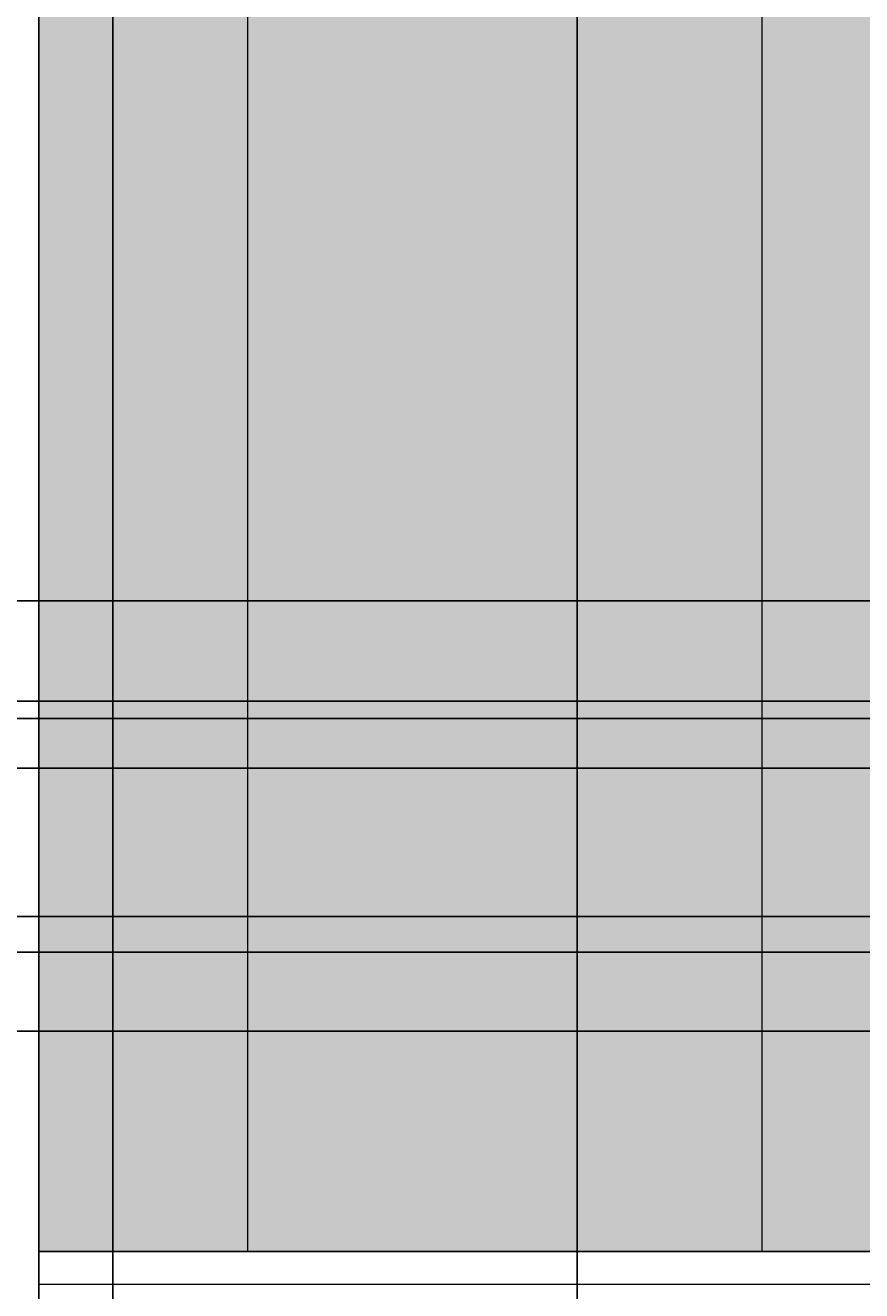
# Model space of a CAD drawing. Units: inches. Extents: x 36 to 594, y 79 to 831.
# Tile 17 of 30: x 93 to 189, y 446 to 590. Entities that reach past the tile are written whole.
import ezdxf

# ---------------------------------------------------------------- set-up
doc = ezdxf.new("R2010")
doc.units = ezdxf.units.IN
doc.header["$MEASUREMENT"] = 0
for name, color, linetype, lineweight in [('A-ANNO-DIMS', 2, 'Continuous', 18), ('A-ELEV', 7, 'Continuous', 25), ('A-ELEV-PATT', 8, 'Continuous', 13), ('A-GLAZ', 4, 'Continuous', 18)]:
    doc.layers.add(name, color=color, linetype=linetype, lineweight=lineweight)
doc.styles.get("Standard").update_dxf_attribs({"font": 'arial.ttf'})
doc.dimstyles.get("Standard").update_dxf_attribs({"dimtxt": 0.8125, "dimasz": 0.18, "dimexe": 0.18, "dimexo": 0.0625, "dimgap": 0.09, "dimtad": 0, "dimtih": 1, "dimtoh": 1, "dimdec": 4, "dimzin": 0, "dimdsep": 46, "dimlunit": 4, "dimtxsty": 'Standard', "dimcen": 0.09, "dimadec": 0, "dimazin": 0, "dimtfac": 1, "dimtdec": 4, "dimtofl": 0, "dimtmove": 0, "dimatfit": 3, "dimfxl": 1, "dimtolj": 1, "dimtzin": 0, "dimarcsym": 0})

# ---------------------------------------------------------------- blocks, each defined once
blk = doc.blocks.new('*D28')
at = {"layer": 'A-ANNO-DIMS', "color": 0, "lineweight": -2, "transparency": 16777216}
for p, q in [((269.3, 796.05), (37.49, 796.05)), ((37.67, 795.87), (37.67, 455.63)), ((37.67, 114.39), (37.67, 454.62)), ((94.8, 114.21), (37.49, 114.21))]:
    blk.add_line(p, q, dxfattribs=at)
at = {"layer": 'A-ANNO-DIMS', "color": 0, "transparency": 16777216}
for points in [[(37.64, 795.87), (37.7, 795.87), (37.67, 796.05)], [(37.64, 114.39), (37.7, 114.39), (37.67, 114.21)]]:
    blk.add_solid(points, dxfattribs=at)
at = {"layer": 'Defpoints', "color": 0, "transparency": 16777216}
for p in [(37.67, 796.05), (269.36, 796.05), (94.87, 114.21)]:
    blk.add_point(p, dxfattribs=at)
at = {"layer": 'A-ANNO-DIMS', "color": 0, "transparency": 16777216, "insert": (37.67, 455.13), "char_height": 0.812, "attachment_point": 5}
blk.add_mtext('\\A1;681.8', dxfattribs=at)
blk = doc.blocks.new('*D60')
at = {"layer": 'A-ANNO-DIMS', "color": 0, "lineweight": -2, "transparency": 16777216}
for p, q in [((103.34, 286.24), (103.34, 830.73)), ((103.52, 830.55), (128.41, 830.55)), ((156.23, 830.55), (131.33, 830.55)), ((156.41, 264.68), (156.41, 830.73))]:
    blk.add_line(p, q, dxfattribs=at)
at = {"layer": 'A-ANNO-DIMS', "color": 0, "transparency": 16777216}
for points in [[(103.52, 830.58), (103.52, 830.52), (103.34, 830.55)], [(156.23, 830.58), (156.23, 830.52), (156.41, 830.55)]]:
    blk.add_solid(points, dxfattribs=at)
at = {"layer": 'Defpoints', "color": 0, "transparency": 16777216}
for p in [(156.41, 830.55), (103.34, 286.18), (156.41, 264.62)]:
    blk.add_point(p, dxfattribs=at)
at = {"layer": 'A-ANNO-DIMS', "color": 0, "transparency": 16777216, "insert": (129.87, 830.55), "char_height": 0.812, "attachment_point": 5}
blk.add_mtext('\\A1;53.07', dxfattribs=at)
blk = doc.blocks.new('*D61')
at = {"layer": 'A-ANNO-DIMS', "color": 0, "lineweight": -2, "transparency": 16777216}
for p, q in [((156.41, 264.68), (156.41, 830.73)), ((156.59, 830.55), (185.26, 830.55)), ((216.85, 830.55), (188.18, 830.55)), ((217.03, 286.24), (217.03, 830.73))]:
    blk.add_line(p, q, dxfattribs=at)
at = {"layer": 'A-ANNO-DIMS', "color": 0, "transparency": 16777216}
for points in [[(156.59, 830.58), (156.59, 830.52), (156.41, 830.55)], [(216.85, 830.58), (216.85, 830.52), (217.03, 830.55)]]:
    blk.add_solid(points, dxfattribs=at)
at = {"layer": 'Defpoints', "color": 0, "transparency": 16777216}
for p in [(217.03, 830.55), (217.03, 286.18), (156.41, 264.62)]:
    blk.add_point(p, dxfattribs=at)
at = {"layer": 'A-ANNO-DIMS', "color": 0, "transparency": 16777216, "insert": (186.72, 830.55), "char_height": 0.812, "attachment_point": 5}
blk.add_mtext('\\A1;60.62', dxfattribs=at)
blk = doc.blocks.new('*D99')
at = {"layer": 'A-ANNO-DIMS', "color": 0, "lineweight": -2, "transparency": 16777216}
for p, q in [((236.23, 484.42), (37.49, 484.42)), ((37.67, 484.24), (37.67, 480.42)), ((37.67, 475.59), (37.67, 479.41)), ((232.76, 475.41), (37.49, 475.41))]:
    blk.add_line(p, q, dxfattribs=at)
at = {"layer": 'A-ANNO-DIMS', "color": 0, "transparency": 16777216}
for points in [[(37.64, 484.24), (37.7, 484.24), (37.67, 484.42)], [(37.64, 475.59), (37.7, 475.59), (37.67, 475.41)]]:
    blk.add_solid(points, dxfattribs=at)
at = {"layer": 'Defpoints', "color": 0, "transparency": 16777216}
for p in [(37.67, 484.42), (236.29, 484.42), (232.82, 475.41)]:
    blk.add_point(p, dxfattribs=at)
at = {"layer": 'A-ANNO-DIMS', "color": 0, "transparency": 16777216, "insert": (37.67, 479.92), "char_height": 0.812, "attachment_point": 5}
blk.add_mtext('\\A1;9.005', dxfattribs=at)
blk = doc.blocks.new('*D100')
at = {"layer": 'A-ANNO-DIMS', "color": 0, "lineweight": -2, "transparency": 16777216}
for p, q in [((236.23, 488.49), (37.49, 488.49)), ((37.67, 488.31), (37.67, 486.96)), ((37.67, 484.6), (37.67, 485.95)), ((236.23, 484.42), (37.49, 484.42))]:
    blk.add_line(p, q, dxfattribs=at)
at = {"layer": 'A-ANNO-DIMS', "color": 0, "transparency": 16777216}
for points in [[(37.64, 488.31), (37.7, 488.31), (37.67, 488.49)], [(37.64, 484.6), (37.7, 484.6), (37.67, 484.42)]]:
    blk.add_solid(points, dxfattribs=at)
at = {"layer": 'Defpoints', "color": 0, "transparency": 16777216}
for p in [(37.67, 488.49), (236.29, 488.49), (236.29, 484.42)]:
    blk.add_point(p, dxfattribs=at)
at = {"layer": 'A-ANNO-DIMS', "color": 0, "transparency": 16777216, "insert": (37.67, 486.46), "char_height": 0.812, "attachment_point": 5}
blk.add_mtext('\\A1;4.074', dxfattribs=at)
blk = doc.blocks.new('*D101')
at = {"layer": 'A-ANNO-DIMS', "color": 0, "lineweight": -2, "transparency": 16777216}
for p, q in [((236.23, 505.45), (37.49, 505.45)), ((37.67, 505.27), (37.67, 497.48)), ((37.67, 488.67), (37.67, 496.47)), ((236.23, 488.49), (37.49, 488.49))]:
    blk.add_line(p, q, dxfattribs=at)
at = {"layer": 'A-ANNO-DIMS', "color": 0, "transparency": 16777216}
for points in [[(37.64, 505.27), (37.7, 505.27), (37.67, 505.45)], [(37.64, 488.67), (37.7, 488.67), (37.67, 488.49)]]:
    blk.add_solid(points, dxfattribs=at)
at = {"layer": 'Defpoints', "color": 0, "transparency": 16777216}
for p in [(37.67, 505.45), (236.29, 505.45), (236.29, 488.49)]:
    blk.add_point(p, dxfattribs=at)
at = {"layer": 'A-ANNO-DIMS', "color": 0, "transparency": 16777216, "insert": (37.67, 496.97), "char_height": 0.812, "attachment_point": 5}
blk.add_mtext('\\A1;16.957', dxfattribs=at)
blk = doc.blocks.new('*D102')
at = {"layer": 'A-ANNO-DIMS', "color": 0, "lineweight": -2, "transparency": 16777216}
for p, q in [((232.76, 511.12), (37.49, 511.12)), ((37.67, 510.94), (37.67, 508.79)), ((37.67, 505.63), (37.67, 507.78)), ((236.23, 505.45), (37.49, 505.45))]:
    blk.add_line(p, q, dxfattribs=at)
at = {"layer": 'A-ANNO-DIMS', "color": 0, "transparency": 16777216}
for points in [[(37.64, 510.94), (37.7, 510.94), (37.67, 511.12)], [(37.64, 505.63), (37.7, 505.63), (37.67, 505.45)]]:
    blk.add_solid(points, dxfattribs=at)
at = {"layer": 'Defpoints', "color": 0, "transparency": 16777216}
for p in [(37.67, 511.12), (232.82, 511.12), (236.29, 505.45)]:
    blk.add_point(p, dxfattribs=at)
at = {"layer": 'A-ANNO-DIMS', "color": 0, "transparency": 16777216, "insert": (37.67, 508.29), "char_height": 0.812, "attachment_point": 5}
blk.add_mtext('\\A1;5.672', dxfattribs=at)
blk = doc.blocks.new('*D103')
at = {"layer": 'A-ANNO-DIMS', "color": 0, "lineweight": -2, "transparency": 16777216}
for p, q in [((232.76, 513.12), (37.49, 513.12)), ((37.67, 512.94), (37.67, 512.62)), ((232.76, 511.12), (37.49, 511.12)), ((37.67, 511.3), (37.67, 511.62))]:
    blk.add_line(p, q, dxfattribs=at)
at = {"layer": 'A-ANNO-DIMS', "color": 0, "transparency": 16777216}
for points in [[(37.64, 512.94), (37.7, 512.94), (37.67, 513.12)], [(37.64, 511.3), (37.7, 511.3), (37.67, 511.12)]]:
    blk.add_solid(points, dxfattribs=at)
at = {"layer": 'Defpoints', "color": 0, "transparency": 16777216}
for p in [(37.67, 513.12), (232.82, 513.12), (232.82, 511.12)]:
    blk.add_point(p, dxfattribs=at)
at = {"layer": 'A-ANNO-DIMS', "color": 0, "transparency": 16777216, "insert": (37.67, 512.12), "char_height": 0.812, "attachment_point": 5}
blk.add_mtext('\\A1;2', dxfattribs=at)
blk = doc.blocks.new('*D104')
at = {"layer": 'A-ANNO-DIMS', "color": 0, "lineweight": -2, "transparency": 16777216}
for p, q in [((232.76, 524.6), (37.49, 524.6)), ((37.67, 524.42), (37.67, 519.37)), ((37.67, 513.3), (37.67, 518.36)), ((232.76, 513.12), (37.49, 513.12))]:
    blk.add_line(p, q, dxfattribs=at)
at = {"layer": 'A-ANNO-DIMS', "color": 0, "transparency": 16777216}
for points in [[(37.64, 524.42), (37.7, 524.42), (37.67, 524.6)], [(37.64, 513.3), (37.7, 513.3), (37.67, 513.12)]]:
    blk.add_solid(points, dxfattribs=at)
at = {"layer": 'Defpoints', "color": 0, "transparency": 16777216}
for p in [(37.67, 524.6), (232.82, 524.6), (232.82, 513.12)]:
    blk.add_point(p, dxfattribs=at)
at = {"layer": 'A-ANNO-DIMS', "color": 0, "transparency": 16777216, "insert": (37.67, 518.86), "char_height": 0.812, "attachment_point": 5}
blk.add_mtext('\\A1;11.481', dxfattribs=at)

msp = doc.modelspace()

# ---------------------------------------------------------------- hatches: boundary and pattern name
at = {"layer": 'A-ELEV-PATT'}
h = msp.add_hatch(color=256, dxfattribs=at)
h.dxf.hatch_style = 1
h.paths.add_polyline_path([(398.0873, 796.0465), (269.3592, 796.0465), (269.3592, 770.1455), (397.8159, 770.1455)])
h.paths.add_polyline_path([(397.7518, 764.0341), (269.3592, 764.0341), (269.3592, 630.0394), (341.8367, 630.0394), (341.8367, 720.595), (335.0881, 728.3699), (329.982, 735.3373), (345.3661, 727.7743), (397.1052, 702.3389)])
h.paths.add_polyline_path([(341.8367, 594.2124), (201.4189, 594.2124), (201.4189, 475.4136), (232.8216, 475.4136), (232.8216, 524.6037), (341.8367, 524.6037)])
h.paths.add_polyline_path([(177.525, 594.2124), (118.7598, 594.2124), (118.7598, 450.2124), (177.525, 450.2124)])
h.paths.add_polyline_path([(424.4958, 594.2124), (365.7306, 594.2124), (365.7306, 450.2124), (424.4958, 450.2124)])
h.paths.add_polyline_path([(241.3553, 404.2737), (355.8569, 404.2737), (355.8569, 355.0836), (424.5492, 355.0836), (424.5492, 425.7333), (118.7598, 426.2844), (118.7598, 355.0836), (241.3553, 355.0836)])
h.paths.add_polyline_path([(448.3898, 306.2124), (217.0273, 306.2124), (217.0273, 142.2124), (254.0293, 142.2124), (254.0293, 150.9347), (254.0293, 286.1802), (401.5491, 286.1802), (401.5491, 150.9347), (401.5491, 142.2124), (448.3898, 142.2124)])
h.paths.add_polyline_path([(448.3898, 142.2124), (401.5491, 142.2124), (217.0273, 142.2124), (217.0273, 114.2124), (448.3898, 114.2124)])
h.paths.add_polyline_path([(217.0273, 306.2124), (174.7353, 306.2124), (94.8658, 306.2124), (94.8658, 162.2124), (103.3368, 162.2124), (103.3368, 264.6224), (103.3368, 286.1802), (217.0273, 286.1802)])
h = msp.add_hatch(color=256, dxfattribs=at)
h.dxf.hatch_style = 1
h.paths.add_polyline_path([(448.3898, 668.2124), (341.8367, 720.595), (341.8367, 594.2124), (341.8367, 450.2124), (365.7306, 450.2124), (365.7306, 594.2124), (424.4958, 594.2124), (424.4958, 450.2124), (448.3898, 450.2124), (448.3898, 594.2124)])
h.paths.add_polyline_path([(378.5958, 653.8563, -1), (413.2033, 653.8563, -1)], flags=16)
h.paths.add_polyline_path([(394.8995, 653.8563), (394.8995, 654.8563), (395.8995, 654.8563), (396.8995, 654.8563), (396.8995, 653.8563), (396.8995, 652.8563), (395.8995, 652.8563), (394.8995, 652.8563)], flags=0)
h.paths.add_polyline_path([(201.4189, 708.8485), (201.4189, 720.595), (94.8658, 668.2124), (94.8658, 644.2124), (94.8658, 596.2124), (94.8658, 594.2124), (94.8658, 450.2124), (118.7598, 450.2124), (118.7598, 594.2124), (177.525, 594.2124), (177.525, 450.2124), (201.4189, 450.2124), (201.4189, 594.2124)])
h.paths.add_polyline_path([(130.1589, 653.7648, -1), (164.7665, 653.7648, -1)], flags=16)
h.paths.add_polyline_path([(148.4627, 652.7648), (147.4627, 652.7648), (146.4627, 652.7648), (146.4627, 653.7648), (146.4627, 654.7648), (147.4627, 654.7648), (148.4627, 654.7648), (148.4627, 653.7648)], flags=0)
h = msp.add_hatch(dxfattribs=at)
h.set_pattern_fill('ANSI31', color=256, scale=38, angle=135)
h.paths.add_polyline_path([(448.3898, 450.2124), (94.8658, 450.2124), (94.8658, 306.2124), (174.7353, 306.2124), (448.3898, 306.2124), (448.3898, 367.5118)])
h.paths.add_polyline_path([(424.5492, 425.7333), (424.5492, 329.5325), (118.7598, 330.0836), (118.7598, 354.0836), (118.7598, 426.2844)], flags=16)
h.paths.add_polyline_path([(355.8569, 404.2737), (355.8569, 355.0836), (241.3553, 355.0836), (241.3553, 404.2737)], flags=0)
h.paths.add_polyline_path([(269.0393, 390.7924), (269.0393, 355.0836), (244.8248, 355.0836), (244.8248, 364.0887), (263.8892, 364.0887), (263.8892, 355.0836), (267.0393, 355.0836), (267.0393, 390.7924)], flags=0)
h.paths.add_polyline_path([(303.9765, 436.9126, -1), (313.1496, 436.9126, -1)], flags=16)
h.paths.add_polyline_path([(421.9473, 354.0836), (421.9376, 348.6883), (421.9376, 333.9204), (401.6342, 333.9204), (401.6705, 354.0836), (400.6705, 354.0836), (400.6608, 348.7267), (400.6608, 333.9587), (380.3574, 333.9587), (380.3937, 354.0836), (379.3937, 354.0836), (379.3841, 348.765), (379.3841, 333.997), (359.0807, 333.997), (359.1169, 354.0836), (358.1169, 354.0836), (358.1074, 348.8034), (358.1074, 334.0354), (337.804, 334.0354), (337.8401, 354.0836), (336.8401, 354.0836), (336.8306, 348.8417), (336.8306, 334.0737), (316.5272, 334.0737), (316.5633, 354.0836), (315.5633, 354.0836), (315.5539, 348.8801), (315.5539, 334.1121), (295.2505, 334.1121), (295.2865, 354.0836), (294.2865, 354.0836), (294.2772, 348.9184), (294.2772, 334.1504), (273.9738, 334.1504), (274.0097, 354.0836), (273.0097, 354.0836), (273.0005, 348.9568), (273.0005, 334.1888), (252.697, 334.1888), (252.7329, 354.0836), (251.7329, 354.0836), (251.7237, 348.9951), (251.7237, 334.2271), (231.4203, 334.2271), (231.4561, 354.0836), (230.4561, 354.0836), (230.447, 349.0335), (230.447, 334.2655), (210.1436, 334.2655), (210.1793, 354.0836), (209.1793, 354.0836), (209.1703, 349.0718), (209.1703, 334.3038), (188.8668, 334.3038), (188.9025, 354.0836), (187.9025, 354.0836), (187.8935, 349.1101), (187.8935, 334.3422), (167.5901, 334.3422), (167.6257, 354.0836), (166.6257, 354.0836), (166.6168, 349.1485), (166.6168, 334.3805), (146.3134, 334.3805), (146.3489, 354.0836), (145.3489, 354.0836), (145.3401, 349.1868), (145.3401, 334.4189), (125.0366, 334.4189), (125.0721, 354.0836)], flags=0)
h.paths.add_polyline_path([(266.285, 436.9126, -1), (275.458, 436.9126, -1)], flags=16)
h.paths.add_polyline_path([(367.0204, 316.8739, -1), (357.8474, 316.8739, -1)], flags=16)
h.paths.add_polyline_path([(347.6933, 316.8739, -1), (338.5202, 316.8739, -1)], flags=16)
h.paths.add_polyline_path([(329.574, 316.8739, -1), (320.401, 316.8739, -1)], flags=16)
h.paths.add_polyline_path([(263.8892, 385.1199), (263.8892, 368.1628), (244.8248, 368.1628), (244.8248, 385.1199)], flags=0)
h.paths.add_polyline_path([(216.2543, 436.9126, -1), (225.4274, 436.9126, -1)], flags=16)
h.paths.add_polyline_path([(275.458, 316.8739, -1), (266.285, 316.8739, -1)], flags=16)
h.paths.add_polyline_path([(225.4274, 316.8739, -1), (216.2543, 316.8739, -1)], flags=16)

# ---------------------------------------------------------------- linework, layer by layer
at = {"layer": 'A-ELEV'}
for p, q in [((94.8658, 450.2124), (94.8658, 594.2124)), ((94.8658, 306.2124), (94.8658, 450.2124)), ((94.8658, 450.2124), (448.3898, 450.2124))]:
    msp.add_line(p, q, dxfattribs=at)
at = {"layer": 'A-GLAZ'}
for p, q in [((118.7598, 450.2124), (118.7598, 594.2124)), ((177.525, 450.2124), (177.525, 594.2124))]:
    msp.add_line(p, q, dxfattribs=at)

# ---------------------------------------------------------------- dimensions: what is measured, and where the dimension line sits
at = {"layer": 'A-ANNO-DIMS'}
for base, p1, p2, picture, middle in [((156.4069, 830.5465), (103.3368, 286.1802), (156.4069, 264.6224), '*D60', (129.8718, 830.5465)), ((217.0273, 830.5465), (156.4069, 264.6224), (217.0273, 286.1802), '*D61', (186.7171, 830.5465))]:
    dim = msp.add_linear_dim(base=base, p1=p1, p2=p2, dimstyle='Standard', override={"dimdec": 2, "dimlfac": 1, "dimrnd": 0, "dimzin": 0, "dimdsep": 46, "dimlunit": 2}, dxfattribs=at)
    dim.commit()
    dim.dimension.update_dxf_attribs({"geometry": picture, "text_midpoint": middle})
for base, p1, p2, override, picture, middle in [((37.6733, 796.0465), (94.8658, 114.2124), (269.3592, 796.0465), {"dimdec": 1, "dimlfac": 1, "dimrnd": 0, "dimzin": 0, "dimdsep": 46, "dimlunit": 2}, '*D28', (37.6733, 455.1294)), ((37.6733, 524.6037), (232.8216, 513.1224), (232.8216, 524.6037), {"dimdec": 3, "dimlfac": 1, "dimrnd": 0, "dimzin": 0, "dimdsep": 46, "dimlunit": 2}, '*D104', (37.6733, 518.863)), ((37.6733, 513.1224), (232.8216, 511.1224), (232.8216, 513.1224), {"dimdec": 0, "dimlfac": 1, "dimrnd": 0, "dimzin": 0, "dimdsep": 46, "dimlunit": 2}, '*D103', (37.6733, 512.1224)), ((37.67335, 511.12236), (236.29105, 505.44988), (232.82156, 511.12236), {"dimdec": 3, "dimlfac": 1, "dimrnd": 0, "dimzin": 0, "dimdsep": 46, "dimlunit": 2}, '*D102', (37.67335, 508.28612)), ((37.6733, 505.4499), (236.2911, 488.4928), (236.2911, 505.4499), {"dimdec": 3, "dimlfac": 1, "dimrnd": 0, "dimzin": 0, "dimdsep": 46, "dimlunit": 2}, '*D101', (37.6733, 496.9714)), ((37.6733, 488.4928), (236.2911, 484.4187), (236.2911, 488.4928), {"dimdec": 3, "dimlfac": 1, "dimrnd": 0, "dimzin": 0, "dimdsep": 46, "dimlunit": 2}, '*D100', (37.6733, 486.4558)), ((37.6733, 484.4187), (232.8216, 475.4136), (236.2911, 484.4187), {"dimdec": 3, "dimlfac": 1, "dimrnd": 0, "dimzin": 0, "dimdsep": 46, "dimlunit": 2}, '*D99', (37.6733, 479.9162))]:
    dim = msp.add_linear_dim(base=base, p1=p1, p2=p2, angle=90, dimstyle='Standard', override=override, dxfattribs=at)
    dim.commit()
    dim.dimension.update_dxf_attribs({"geometry": picture, "text_midpoint": middle})

doc.saveas('drawing.dxf')
